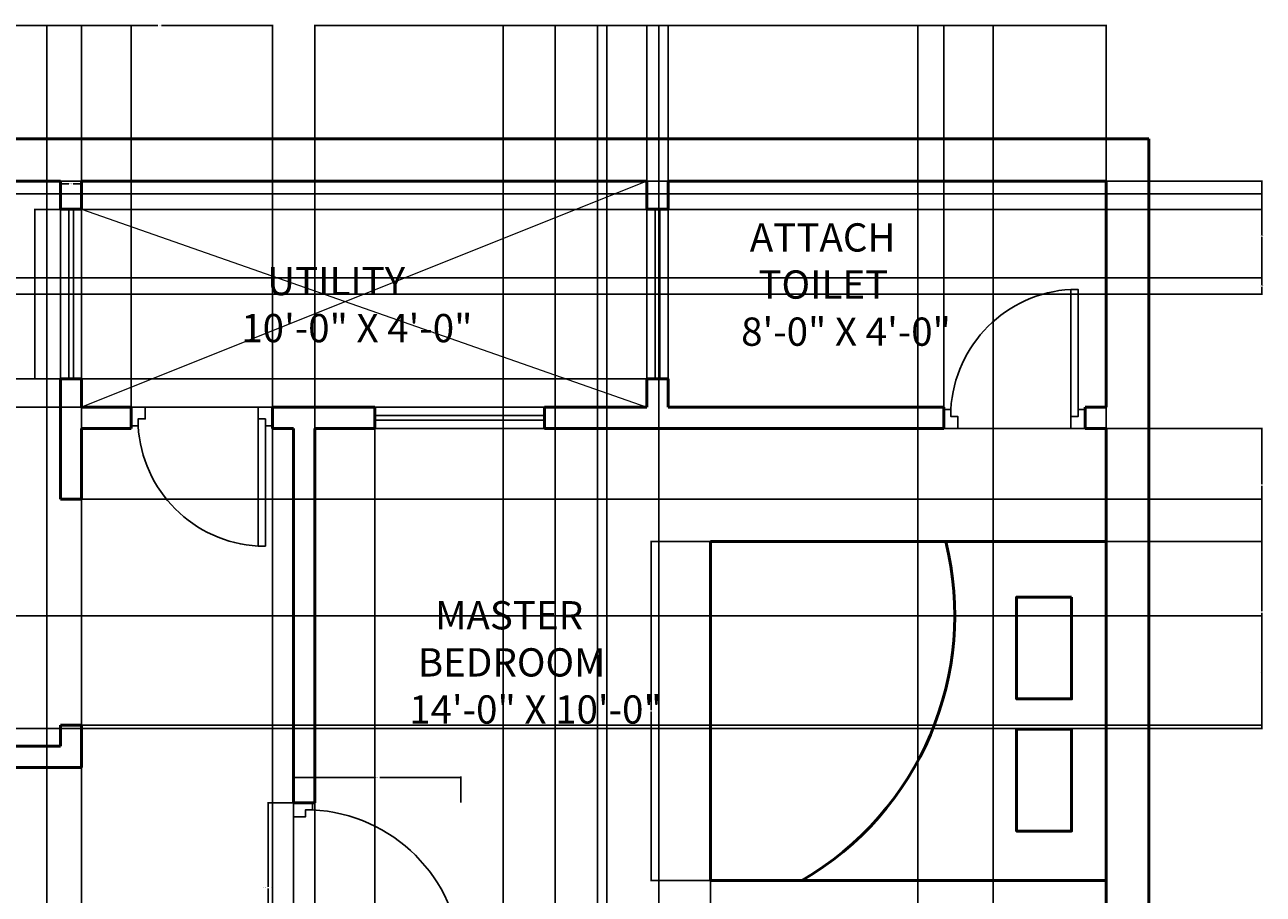
# Model space of a CAD drawing. Units: inches. Extents: x 2330 to 2739, y 947 to 1475.
# Tile 6 of 6: x 2476 to 2739, y 1291 to 1475. Entities that reach past the tile are written whole.
import ezdxf

# ---------------------------------------------------------------- set-up
doc = ezdxf.new("R2010")
doc.units = ezdxf.units.IN
for name, color, linetype, lineweight in [('A-ANNO-DIMS', 2, 'Continuous', 18), ('A-AREA-IDEN', 7, 'Continuous', 25), ('door', 150, 'Continuous', 25), ('furniture', 9, 'Continuous', 18), ('railing', 224, 'Continuous', 13), ('wall', 7, 'Continuous', 50), ('window', 40, 'Continuous', 25)]:
    doc.layers.add(name, color=color, linetype=linetype, lineweight=lineweight)
doc.styles.get("Standard").update_dxf_attribs({"font": 'arial.ttf'})
doc.dimstyles.get("Standard").update_dxf_attribs({"dimtxt": 0.18, "dimasz": 0.18, "dimexe": 0.18, "dimexo": 0.0625, "dimgap": 0.09, "dimtad": 0, "dimtih": 1, "dimtoh": 1, "dimdec": 4, "dimzin": 0, "dimdsep": 46, "dimtxsty": 'Standard', "dimcen": 0.09, "dimadec": 0, "dimazin": 0, "dimtfac": 1, "dimtdec": 4, "dimtofl": 0, "dimtmove": 0, "dimatfit": 3, "dimfxl": 1, "dimtolj": 1, "dimtzin": 0, "dimarcsym": 0})

# ---------------------------------------------------------------- blocks, each defined once
blk = doc.blocks.new('w3')
at = {"layer": 'window'}
for p, q in [((2833.35, 1386.77), (2833.35, 1350.77)), ((2834.35, 1386.77), (2834.35, 1350.77))]:
    blk.add_line(p, q, dxfattribs=at)
blk.add_lwpolyline([(2831.6, 1350.77), (2836.1, 1350.77), (2836.1, 1386.77), (2831.6, 1386.77)], close=True, dxfattribs=at)
blk = doc.blocks.new('d1')
at = {"layer": 'door'}
blk.add_line((2897.27, 1313.4), (2933.27, 1313.4), dxfattribs=at)
blk.add_lwpolyline([(2898.77, 1315.9), (2900.27, 1315.9), (2900.27, 1348.9), (2898.77, 1348.9)], close=True, dxfattribs=at)
for points in [[(2900.27, 1313.4), (2897.27, 1313.4), (2897.27, 1317.4), (2898.77, 1317.4), (2898.77, 1315.9), (2900.27, 1315.9), (2900.27, 1313.4)], [(2930.27, 1313.4), (2933.27, 1313.4), (2933.27, 1317.4), (2931.77, 1317.4), (2931.77, 1315.9), (2930.27, 1315.9), (2930.27, 1313.4)]]:
    blk.add_lwpolyline(points, dxfattribs=at)
blk.add_arc((2898.77, 1315.9), 33.03, 2.6026, 87.3974, dxfattribs=at)
blk = doc.blocks.new('d2')
at = {"layer": 'door'}
blk.add_line((2897.27, 1250.29), (2927.27, 1250.29), dxfattribs=at)
blk.add_lwpolyline([(2898.77, 1252.79), (2900.27, 1252.79), (2900.27, 1279.79), (2898.77, 1279.79)], close=True, dxfattribs=at)
for points in [[(2900.27, 1250.29), (2897.27, 1250.29), (2897.27, 1254.29), (2898.77, 1254.29), (2898.77, 1252.79), (2900.27, 1252.79), (2900.27, 1250.29)], [(2924.27, 1250.29), (2927.27, 1250.29), (2927.27, 1254.29), (2925.77, 1254.29), (2925.77, 1252.79), (2924.27, 1252.79), (2924.27, 1250.29)]]:
    blk.add_lwpolyline(points, dxfattribs=at)
blk.add_arc((2898.77, 1252.79), 27.04, 3.1798, 86.8202, dxfattribs=at)
blk = doc.blocks.new('BED')
at = {"layer": 'wall'}
for points in [[(2902.88, 1364.87), (2974.88, 1364.87), (2974.88, 1448.87), (2902.88, 1448.87)], [(2914.71, 1441.49), (2936.34, 1441.49), (2936.34, 1429.82), (2914.71, 1429.82)], [(2942.76, 1441.49), (2964.39, 1441.49), (2964.39, 1429.82), (2942.76, 1429.82)]]:
    blk.add_lwpolyline(points, close=True, dxfattribs=at)
blk.add_arc((2918.5, 1351.51), 65.2, 30.1485, 103.8594, dxfattribs=at)
blk = doc.blocks.new('*D10')
at = {"layer": 'A-ANNO-DIMS', "color": 0, "lineweight": -2, "transparency": 16777216}
for p, q in [((2483.62, 1436.28), (2478.1, 1436.28)), ((2478.28, 1436.1), (2478.28, 1418.47)), ((2478.28, 1400.46), (2478.28, 1418.1)), ((2483.62, 1400.28), (2478.1, 1400.28))]:
    blk.add_line(p, q, dxfattribs=at)
at = {"layer": 'A-ANNO-DIMS', "color": 0, "transparency": 16777216}
for points in [[(2478.25, 1436.1), (2478.31, 1436.1), (2478.28, 1436.28)], [(2478.25, 1400.46), (2478.31, 1400.46), (2478.28, 1400.28)]]:
    blk.add_solid(points, dxfattribs=at)
at = {"layer": 'Defpoints', "color": 0, "transparency": 16777216}
for p in [(2478.28, 1436.28), (2483.68, 1436.28), (2483.68, 1400.28)]:
    blk.add_point(p, dxfattribs=at)
at = {"layer": 'A-ANNO-DIMS', "color": 0, "transparency": 16777216, "insert": (2478.28, 1418.28), "char_height": 0.18, "attachment_point": 5}
blk.add_mtext('\\A1;WINDOW W3 36 TYP.', dxfattribs=at)
blk = doc.blocks.new('*D11')
at = {"layer": 'A-ANNO-DIMS', "color": 0, "lineweight": -2, "transparency": 16777216}
for p, q in [((2483.68, 1436.34), (2483.68, 1441.86)), ((2483.86, 1441.68), (2485.47, 1441.68)), ((2488, 1441.68), (2486.39, 1441.68)), ((2488.18, 1436.34), (2488.18, 1441.86))]:
    blk.add_line(p, q, dxfattribs=at)
at = {"layer": 'A-ANNO-DIMS', "color": 0, "transparency": 16777216}
for points in [[(2483.86, 1441.71), (2483.86, 1441.65), (2483.68, 1441.68)], [(2488, 1441.71), (2488, 1441.65), (2488.18, 1441.68)]]:
    blk.add_solid(points, dxfattribs=at)
at = {"layer": 'Defpoints', "color": 0, "transparency": 16777216}
for p in [(2488.18, 1441.68), (2483.68, 1436.28), (2488.18, 1436.28)]:
    blk.add_point(p, dxfattribs=at)
at = {"layer": 'A-ANNO-DIMS', "color": 0, "transparency": 16777216, "insert": (2485.93, 1441.68), "char_height": 0.18, "attachment_point": 5}
blk.add_mtext('\\A1;5 TYP.', dxfattribs=at)
blk = doc.blocks.new('*D16')
at = {"layer": 'A-ANNO-DIMS', "color": 0, "lineweight": -2, "transparency": 16777216}
for p, q in [((2533.12, 1310.28), (2527.6, 1310.28)), ((2527.78, 1310.1), (2527.78, 1292.47)), ((2527.78, 1274.46), (2527.78, 1292.1)), ((2533.12, 1274.28), (2527.6, 1274.28))]:
    blk.add_line(p, q, dxfattribs=at)
at = {"layer": 'A-ANNO-DIMS', "color": 0, "transparency": 16777216}
for points in [[(2527.75, 1310.1), (2527.81, 1310.1), (2527.78, 1310.28)], [(2527.75, 1274.46), (2527.81, 1274.46), (2527.78, 1274.28)]]:
    blk.add_solid(points, dxfattribs=at)
at = {"layer": 'Defpoints', "color": 0, "transparency": 16777216}
for p in [(2527.78, 1310.28), (2533.18, 1310.28), (2533.18, 1274.28)]:
    blk.add_point(p, dxfattribs=at)
at = {"layer": 'A-ANNO-DIMS', "color": 0, "transparency": 16777216, "insert": (2527.78, 1292.28), "char_height": 0.18, "attachment_point": 5}
blk.add_mtext('\\A1;DOOR D1 36 TYP.', dxfattribs=at)
blk = doc.blocks.new('*D17')
at = {"layer": 'A-ANNO-DIMS', "color": 0, "lineweight": -2, "transparency": 16777216}
for p, q in [((2533.18, 1310.34), (2533.18, 1315.86)), ((2533.36, 1315.68), (2550.4, 1315.68)), ((2568.5, 1315.68), (2551.46, 1315.68)), ((2568.68, 1310.34), (2568.68, 1315.86))]:
    blk.add_line(p, q, dxfattribs=at)
at = {"layer": 'A-ANNO-DIMS', "color": 0, "transparency": 16777216}
for points in [[(2533.36, 1315.71), (2533.36, 1315.65), (2533.18, 1315.68)], [(2568.5, 1315.71), (2568.5, 1315.65), (2568.68, 1315.68)]]:
    blk.add_solid(points, dxfattribs=at)
at = {"layer": 'Defpoints', "color": 0, "transparency": 16777216}
for p in [(2568.68, 1315.68), (2533.18, 1310.28), (2568.68, 1310.28)]:
    blk.add_point(p, dxfattribs=at)
at = {"layer": 'A-ANNO-DIMS', "color": 0, "transparency": 16777216, "insert": (2550.93, 1315.68), "char_height": 0.18, "attachment_point": 5}
blk.add_mtext('\\A1;36 TYP.', dxfattribs=at)
blk = doc.blocks.new('*D18')
at = {"layer": 'A-ANNO-DIMS', "color": 0, "lineweight": -2, "transparency": 16777216}
for p, q in [((2621.68, 1293.72), (2621.68, 1281)), ((2705.68, 1293.72), (2705.68, 1281)), ((2621.86, 1281.18), (2662.86, 1281.18)), ((2705.5, 1281.18), (2664.5, 1281.18))]:
    blk.add_line(p, q, dxfattribs=at)
at = {"layer": 'A-ANNO-DIMS', "color": 0, "transparency": 16777216}
for points in [[(2621.86, 1281.21), (2621.86, 1281.15), (2621.68, 1281.18)], [(2705.5, 1281.21), (2705.5, 1281.15), (2705.68, 1281.18)]]:
    blk.add_solid(points, dxfattribs=at)
at = {"layer": 'Defpoints', "color": 0, "transparency": 16777216}
for p in [(2621.68, 1293.78), (2705.68, 1293.78), (2705.68, 1281.18)]:
    blk.add_point(p, dxfattribs=at)
at = {"layer": 'A-ANNO-DIMS', "color": 0, "transparency": 16777216, "insert": (2663.68, 1281.18), "char_height": 0.18, "attachment_point": 5}
blk.add_mtext('\\A1;BED 84 TYP.', dxfattribs=at)
blk = doc.blocks.new('*D19')
at = {"layer": 'A-ANNO-DIMS', "color": 0, "lineweight": -2, "transparency": 16777216}
for p, q in [((2621.62, 1365.78), (2608.9, 1365.78)), ((2609.08, 1365.6), (2609.08, 1329.96)), ((2609.08, 1293.96), (2609.08, 1329.6)), ((2621.62, 1293.78), (2608.9, 1293.78))]:
    blk.add_line(p, q, dxfattribs=at)
at = {"layer": 'A-ANNO-DIMS', "color": 0, "transparency": 16777216}
for points in [[(2609.05, 1365.6), (2609.11, 1365.6), (2609.08, 1365.78)], [(2609.05, 1293.96), (2609.11, 1293.96), (2609.08, 1293.78)]]:
    blk.add_solid(points, dxfattribs=at)
at = {"layer": 'Defpoints', "color": 0, "transparency": 16777216}
for p in [(2621.68, 1365.78), (2609.08, 1293.78), (2621.68, 1293.78)]:
    blk.add_point(p, dxfattribs=at)
at = {"layer": 'A-ANNO-DIMS', "color": 0, "transparency": 16777216, "insert": (2609.08, 1329.78), "char_height": 0.18, "attachment_point": 5}
blk.add_mtext('\\A1;72 TYP.', dxfattribs=at)
blk = doc.blocks.new('*D27')
at = {"layer": 'A-ANNO-DIMS', "color": 0, "lineweight": -2, "transparency": 16777216}
for p, q in [((2537.68, 980.34), (2537.68, 1475.46)), ((2537.86, 1475.28), (2567.46, 1475.28)), ((2597.5, 1475.28), (2567.9, 1475.28)), ((2597.68, 980.34), (2597.68, 1475.46))]:
    blk.add_line(p, q, dxfattribs=at)
at = {"layer": 'A-ANNO-DIMS', "color": 0, "transparency": 16777216}
for points in [[(2537.86, 1475.31), (2537.86, 1475.25), (2537.68, 1475.28)], [(2597.5, 1475.31), (2597.5, 1475.25), (2597.68, 1475.28)]]:
    blk.add_solid(points, dxfattribs=at)
at = {"layer": 'Defpoints', "color": 0, "transparency": 16777216}
for p in [(2597.68, 1475.28), (2537.68, 980.28), (2597.68, 980.28)]:
    blk.add_point(p, dxfattribs=at)
at = {"layer": 'A-ANNO-DIMS', "color": 0, "transparency": 16777216, "insert": (2567.68, 1475.28), "char_height": 0.18, "attachment_point": 5}
blk.add_mtext('\\A1;60', dxfattribs=at)
blk = doc.blocks.new('*D29')
at = {"layer": 'A-ANNO-DIMS', "color": 0, "lineweight": -2, "transparency": 16777216}
for p, q in [((2705.74, 1389.78), (2738.86, 1389.78)), ((2738.68, 1389.6), (2738.68, 1377.96)), ((2738.68, 1365.96), (2738.68, 1377.6)), ((2705.74, 1365.78), (2738.86, 1365.78))]:
    blk.add_line(p, q, dxfattribs=at)
at = {"layer": 'A-ANNO-DIMS', "color": 0, "transparency": 16777216}
for points in [[(2738.65, 1389.6), (2738.71, 1389.6), (2738.68, 1389.78)], [(2738.65, 1365.96), (2738.71, 1365.96), (2738.68, 1365.78)]]:
    blk.add_solid(points, dxfattribs=at)
at = {"layer": 'Defpoints', "color": 0, "transparency": 16777216}
for p in [(2705.68, 1389.78), (2705.68, 1365.78), (2738.68, 1365.78)]:
    blk.add_point(p, dxfattribs=at)
at = {"layer": 'A-ANNO-DIMS', "color": 0, "transparency": 16777216, "insert": (2738.68, 1377.78), "char_height": 0.18, "attachment_point": 5}
blk.add_mtext('\\A1;24', dxfattribs=at)
blk = doc.blocks.new('*D34')
at = {"layer": 'A-ANNO-DIMS', "color": 0, "lineweight": -2, "transparency": 16777216}
for p, q in [((2449.93, 1139.34), (2449.93, 1475.46)), ((2450.11, 1475.28), (2468.66, 1475.28)), ((2488, 1475.28), (2469.45, 1475.28)), ((2488.18, 1139.34), (2488.18, 1475.46))]:
    blk.add_line(p, q, dxfattribs=at)
at = {"layer": 'A-ANNO-DIMS', "color": 0, "transparency": 16777216}
for points in [[(2450.11, 1475.31), (2450.11, 1475.25), (2449.93, 1475.28)], [(2488, 1475.31), (2488, 1475.25), (2488.18, 1475.28)]]:
    blk.add_solid(points, dxfattribs=at)
at = {"layer": 'Defpoints', "color": 0, "transparency": 16777216}
for p in [(2488.18, 1475.28), (2449.93, 1139.28), (2488.18, 1139.28)]:
    blk.add_point(p, dxfattribs=at)
at = {"layer": 'A-ANNO-DIMS', "color": 0, "transparency": 16777216, "insert": (2469.05, 1475.28), "char_height": 0.18, "attachment_point": 5}
blk.add_mtext('\\A1;38.25', dxfattribs=at)
blk = doc.blocks.new('*D35')
at = {"layer": 'A-ANNO-DIMS', "color": 0, "lineweight": -2, "transparency": 16777216}
for p, q in [((2488.18, 1394.34), (2488.18, 1475.46)), ((2488.36, 1475.28), (2493.11, 1475.28)), ((2498.5, 1475.28), (2493.74, 1475.28)), ((2498.68, 1394.34), (2498.68, 1475.46))]:
    blk.add_line(p, q, dxfattribs=at)
at = {"layer": 'A-ANNO-DIMS', "color": 0, "transparency": 16777216}
for points in [[(2488.36, 1475.31), (2488.36, 1475.25), (2488.18, 1475.28)], [(2498.5, 1475.31), (2498.5, 1475.25), (2498.68, 1475.28)]]:
    blk.add_solid(points, dxfattribs=at)
at = {"layer": 'Defpoints', "color": 0, "transparency": 16777216}
for p in [(2498.68, 1475.28), (2488.18, 1394.28), (2498.68, 1394.28)]:
    blk.add_point(p, dxfattribs=at)
at = {"layer": 'A-ANNO-DIMS', "color": 0, "transparency": 16777216, "insert": (2493.43, 1475.28), "char_height": 0.18, "attachment_point": 5}
blk.add_mtext('\\A1;10.5', dxfattribs=at)
blk = doc.blocks.new('*D36')
at = {"layer": 'A-ANNO-DIMS', "color": 0, "lineweight": -2, "transparency": 16777216}
for p, q in [((2528.68, 1394.22), (2528.68, 947.1)), ((2550.43, 1394.22), (2550.43, 947.1)), ((2528.86, 947.28), (2539.16, 947.28)), ((2550.25, 947.28), (2539.95, 947.28))]:
    blk.add_line(p, q, dxfattribs=at)
at = {"layer": 'A-ANNO-DIMS', "color": 0, "transparency": 16777216}
for points in [[(2528.86, 947.31), (2528.86, 947.25), (2528.68, 947.28)], [(2550.25, 947.31), (2550.25, 947.25), (2550.43, 947.28)]]:
    blk.add_solid(points, dxfattribs=at)
at = {"layer": 'Defpoints', "color": 0, "transparency": 16777216}
for p in [(2528.68, 1394.28), (2550.43, 1394.28), (2550.43, 947.28)]:
    blk.add_point(p, dxfattribs=at)
at = {"layer": 'A-ANNO-DIMS', "color": 0, "transparency": 16777216, "insert": (2539.55, 947.28), "char_height": 0.18, "attachment_point": 5}
blk.add_mtext('\\A1;21.75', dxfattribs=at)
blk = doc.blocks.new('*D37')
at = {"layer": 'A-ANNO-DIMS', "color": 0, "lineweight": -2, "transparency": 16777216}
for p, q in [((2608.18, 1442.34), (2608.18, 1475.46)), ((2608.36, 1475.28), (2610.17, 1475.28)), ((2612.5, 1475.28), (2610.69, 1475.28)), ((2612.68, 1442.34), (2612.68, 1475.46))]:
    blk.add_line(p, q, dxfattribs=at)
at = {"layer": 'A-ANNO-DIMS', "color": 0, "transparency": 16777216}
for points in [[(2608.36, 1475.31), (2608.36, 1475.25), (2608.18, 1475.28)], [(2612.5, 1475.31), (2612.5, 1475.25), (2612.68, 1475.28)]]:
    blk.add_solid(points, dxfattribs=at)
at = {"layer": 'Defpoints', "color": 0, "transparency": 16777216}
for p in [(2608.18, 1475.28), (2608.18, 1442.28), (2612.68, 1442.28)]:
    blk.add_point(p, dxfattribs=at)
at = {"layer": 'A-ANNO-DIMS', "color": 0, "transparency": 16777216, "insert": (2610.43, 1475.28), "char_height": 0.18, "attachment_point": 5}
blk.add_mtext('\\A1;4.5', dxfattribs=at)
blk = doc.blocks.new('*D38')
at = {"layer": 'A-ANNO-DIMS', "color": 0, "lineweight": -2, "transparency": 16777216}
for p, q in [((2537.68, 1134.84), (2537.68, 1475.46)), ((2537.86, 1475.28), (2562.98, 1475.28)), ((2588.5, 1475.28), (2563.38, 1475.28)), ((2588.68, 1134.84), (2588.68, 1475.46))]:
    blk.add_line(p, q, dxfattribs=at)
at = {"layer": 'A-ANNO-DIMS', "color": 0, "transparency": 16777216}
for points in [[(2537.86, 1475.31), (2537.86, 1475.25), (2537.68, 1475.28)], [(2588.5, 1475.31), (2588.5, 1475.25), (2588.68, 1475.28)]]:
    blk.add_solid(points, dxfattribs=at)
at = {"layer": 'Defpoints', "color": 0, "transparency": 16777216}
for p in [(2588.68, 1475.28), (2537.68, 1134.78), (2588.68, 1134.78)]:
    blk.add_point(p, dxfattribs=at)
at = {"layer": 'A-ANNO-DIMS', "color": 0, "transparency": 16777216, "insert": (2563.18, 1475.28), "char_height": 0.18, "attachment_point": 5}
blk.add_mtext('\\A1;51', dxfattribs=at)
blk = doc.blocks.new('*D41')
at = {"layer": 'A-ANNO-DIMS', "color": 0, "lineweight": -2, "transparency": 16777216}
for p, q in [((2612.68, 1394.34), (2612.68, 1475.46)), ((2612.86, 1475.28), (2641.6, 1475.28)), ((2671, 1475.28), (2642.25, 1475.28)), ((2671.18, 1394.34), (2671.18, 1475.46))]:
    blk.add_line(p, q, dxfattribs=at)
at = {"layer": 'A-ANNO-DIMS', "color": 0, "transparency": 16777216}
for points in [[(2612.86, 1475.31), (2612.86, 1475.25), (2612.68, 1475.28)], [(2671, 1475.31), (2671, 1475.25), (2671.18, 1475.28)]]:
    blk.add_solid(points, dxfattribs=at)
at = {"layer": 'Defpoints', "color": 0, "transparency": 16777216}
for p in [(2612.68, 1475.28), (2612.68, 1394.28), (2671.18, 1394.28)]:
    blk.add_point(p, dxfattribs=at)
at = {"layer": 'A-ANNO-DIMS', "color": 0, "transparency": 16777216, "insert": (2641.93, 1475.28), "char_height": 0.18, "attachment_point": 5}
blk.add_mtext('\\A1;58.5', dxfattribs=at)
blk = doc.blocks.new('*D62')
at = {"layer": 'A-ANNO-DIMS', "color": 0, "lineweight": -2, "transparency": 16777216}
for p, q in [((2426.7, 1439.54), (2738.86, 1439.54)), ((2738.68, 1439.36), (2738.68, 1430.83)), ((2738.68, 1421.95), (2738.68, 1430.47)), ((2426.7, 1421.77), (2738.86, 1421.77))]:
    blk.add_line(p, q, dxfattribs=at)
at = {"layer": 'A-ANNO-DIMS', "color": 0, "transparency": 16777216}
for points in [[(2738.65, 1439.36), (2738.71, 1439.36), (2738.68, 1439.54)], [(2738.65, 1421.95), (2738.71, 1421.95), (2738.68, 1421.77)]]:
    blk.add_solid(points, dxfattribs=at)
at = {"layer": 'Defpoints', "color": 0, "transparency": 16777216}
for p in [(2426.64, 1439.54), (2738.68, 1439.54), (2426.64, 1421.77)]:
    blk.add_point(p, dxfattribs=at)
at = {"layer": 'A-ANNO-DIMS', "color": 0, "transparency": 16777216, "insert": (2738.68, 1430.65), "char_height": 0.18, "attachment_point": 5}
blk.add_mtext('\\A1;17.77', dxfattribs=at)
blk = doc.blocks.new('*D64')
at = {"layer": 'A-ANNO-DIMS', "color": 0, "lineweight": -2, "transparency": 16777216}
for p, q in [((2426.7, 1421.77), (2738.86, 1421.77)), ((2738.68, 1421.59), (2738.68, 1420.21)), ((2738.68, 1418.46), (2738.68, 1419.84)), ((2443.26, 1418.28), (2738.86, 1418.28))]:
    blk.add_line(p, q, dxfattribs=at)
at = {"layer": 'A-ANNO-DIMS', "color": 0, "transparency": 16777216}
for points in [[(2738.65, 1421.59), (2738.71, 1421.59), (2738.68, 1421.77)], [(2738.65, 1418.46), (2738.71, 1418.46), (2738.68, 1418.28)]]:
    blk.add_solid(points, dxfattribs=at)
at = {"layer": 'Defpoints', "color": 0, "transparency": 16777216}
for p in [(2426.64, 1421.77), (2443.2, 1418.28), (2738.68, 1418.28)]:
    blk.add_point(p, dxfattribs=at)
at = {"layer": 'A-ANNO-DIMS', "color": 0, "transparency": 16777216, "insert": (2738.68, 1420.03), "char_height": 0.18, "attachment_point": 5}
blk.add_mtext('\\A1;3.487', dxfattribs=at)
blk = doc.blocks.new('*D68')
at = {"layer": 'A-ANNO-DIMS', "color": 0, "lineweight": -2, "transparency": 16777216}
for p, q in [((2483.74, 1374.78), (2738.86, 1374.78)), ((2738.68, 1374.6), (2738.68, 1350.96)), ((2738.68, 1326.96), (2738.68, 1350.6)), ((2483.74, 1326.78), (2738.86, 1326.78))]:
    blk.add_line(p, q, dxfattribs=at)
at = {"layer": 'A-ANNO-DIMS', "color": 0, "transparency": 16777216}
for points in [[(2738.65, 1374.6), (2738.71, 1374.6), (2738.68, 1374.78)], [(2738.65, 1326.96), (2738.71, 1326.96), (2738.68, 1326.78)]]:
    blk.add_solid(points, dxfattribs=at)
at = {"layer": 'Defpoints', "color": 0, "transparency": 16777216}
for p in [(2483.68, 1374.78), (2738.68, 1374.78), (2483.68, 1326.78)]:
    blk.add_point(p, dxfattribs=at)
at = {"layer": 'A-ANNO-DIMS', "color": 0, "transparency": 16777216, "insert": (2738.68, 1350.78), "char_height": 0.18, "attachment_point": 5}
blk.add_mtext('\\A1;48', dxfattribs=at)
blk = doc.blocks.new('*D69')
at = {"layer": 'A-ANNO-DIMS', "color": 0, "lineweight": -2, "transparency": 16777216}
for p, q in [((2483.74, 1442.28), (2738.86, 1442.28)), ((2738.68, 1442.1), (2738.68, 1439.46)), ((2738.68, 1436.46), (2738.68, 1439.1)), ((2483.74, 1436.28), (2738.86, 1436.28))]:
    blk.add_line(p, q, dxfattribs=at)
at = {"layer": 'A-ANNO-DIMS', "color": 0, "transparency": 16777216}
for points in [[(2738.65, 1442.1), (2738.71, 1442.1), (2738.68, 1442.28)], [(2738.65, 1436.46), (2738.71, 1436.46), (2738.68, 1436.28)]]:
    blk.add_solid(points, dxfattribs=at)
at = {"layer": 'Defpoints', "color": 0, "transparency": 16777216}
for p in [(2483.68, 1442.28), (2483.68, 1436.28), (2738.68, 1436.28)]:
    blk.add_point(p, dxfattribs=at)
at = {"layer": 'A-ANNO-DIMS', "color": 0, "transparency": 16777216, "insert": (2738.68, 1439.28), "char_height": 0.18, "attachment_point": 5}
blk.add_mtext('\\A1;6', dxfattribs=at)
blk = doc.blocks.new('*D71')
at = {"layer": 'A-ANNO-DIMS', "color": 0, "lineweight": -2, "transparency": 16777216}
for p, q in [((2392.26, 1349.96), (2738.86, 1349.96)), ((2738.68, 1349.78), (2738.68, 1338.17)), ((2738.68, 1326.21), (2738.68, 1337.81)), ((2392.26, 1326.03), (2738.86, 1326.03))]:
    blk.add_line(p, q, dxfattribs=at)
at = {"layer": 'A-ANNO-DIMS', "color": 0, "transparency": 16777216}
for points in [[(2738.65, 1349.78), (2738.71, 1349.78), (2738.68, 1349.96)], [(2738.65, 1326.21), (2738.71, 1326.21), (2738.68, 1326.03)]]:
    blk.add_solid(points, dxfattribs=at)
at = {"layer": 'Defpoints', "color": 0, "transparency": 16777216}
for p in [(2392.19, 1349.96), (2738.68, 1349.96), (2392.19, 1326.03)]:
    blk.add_point(p, dxfattribs=at)
at = {"layer": 'A-ANNO-DIMS', "color": 0, "transparency": 16777216, "insert": (2738.68, 1337.99), "char_height": 0.18, "attachment_point": 5}
blk.add_mtext('\\A1;23.93', dxfattribs=at)
blk = doc.blocks.new('*D72')
at = {"layer": 'A-ANNO-DIMS', "color": 0, "lineweight": -2, "transparency": 16777216}
for p, q in [((2599.68, 1187.34), (2599.68, 1475.46)), ((2599.86, 1475.28), (2604.99, 1475.28)), ((2610.5, 1475.28), (2605.37, 1475.28)), ((2610.68, 1187.34), (2610.68, 1475.46))]:
    blk.add_line(p, q, dxfattribs=at)
at = {"layer": 'A-ANNO-DIMS', "color": 0, "transparency": 16777216}
for points in [[(2599.86, 1475.31), (2599.86, 1475.25), (2599.68, 1475.28)], [(2610.5, 1475.31), (2610.5, 1475.25), (2610.68, 1475.28)]]:
    blk.add_solid(points, dxfattribs=at)
at = {"layer": 'Defpoints', "color": 0, "transparency": 16777216}
for p in [(2610.68, 1475.28), (2599.68, 1187.28), (2610.68, 1187.28)]:
    blk.add_point(p, dxfattribs=at)
at = {"layer": 'A-ANNO-DIMS', "color": 0, "transparency": 16777216, "insert": (2605.18, 1475.28), "char_height": 0.18, "attachment_point": 5}
blk.add_mtext('\\A1;11', dxfattribs=at)
blk = doc.blocks.new('*D75')
at = {"layer": 'A-ANNO-DIMS', "color": 0, "lineweight": -2, "transparency": 16777216}
for p, q in [((2665.68, 1187.34), (2665.68, 1475.46)), ((2665.86, 1475.28), (2685.46, 1475.28)), ((2705.5, 1475.28), (2685.9, 1475.28)), ((2705.68, 1187.34), (2705.68, 1475.46))]:
    blk.add_line(p, q, dxfattribs=at)
at = {"layer": 'A-ANNO-DIMS', "color": 0, "transparency": 16777216}
for points in [[(2665.86, 1475.31), (2665.86, 1475.25), (2665.68, 1475.28)], [(2705.5, 1475.31), (2705.5, 1475.25), (2705.68, 1475.28)]]:
    blk.add_solid(points, dxfattribs=at)
at = {"layer": 'Defpoints', "color": 0, "transparency": 16777216}
for p in [(2705.68, 1475.28), (2665.68, 1187.28), (2705.68, 1187.28)]:
    blk.add_point(p, dxfattribs=at)
at = {"layer": 'A-ANNO-DIMS', "color": 0, "transparency": 16777216, "insert": (2685.68, 1475.28), "char_height": 0.18, "attachment_point": 5}
blk.add_mtext('\\A1;40', dxfattribs=at)
blk = doc.blocks.new('*D76')
at = {"layer": 'A-ANNO-DIMS', "color": 0, "lineweight": -2, "transparency": 16777216}
for p, q in [((2577.68, 1265.34), (2577.68, 1475.46)), ((2577.86, 1475.28), (2621.46, 1475.28)), ((2665.5, 1475.28), (2621.9, 1475.28)), ((2665.68, 1265.34), (2665.68, 1475.46))]:
    blk.add_line(p, q, dxfattribs=at)
at = {"layer": 'A-ANNO-DIMS', "color": 0, "transparency": 16777216}
for points in [[(2577.86, 1475.31), (2577.86, 1475.25), (2577.68, 1475.28)], [(2665.5, 1475.31), (2665.5, 1475.25), (2665.68, 1475.28)]]:
    blk.add_solid(points, dxfattribs=at)
at = {"layer": 'Defpoints', "color": 0, "transparency": 16777216}
for p in [(2665.68, 1475.28), (2577.68, 1265.28), (2665.68, 1265.28)]:
    blk.add_point(p, dxfattribs=at)
at = {"layer": 'A-ANNO-DIMS', "color": 0, "transparency": 16777216, "insert": (2621.68, 1475.28), "char_height": 0.18, "attachment_point": 5}
blk.add_mtext('\\A1;88', dxfattribs=at)
blk = doc.blocks.new('*D78')
at = {"layer": 'A-ANNO-DIMS', "color": 0, "lineweight": -2, "transparency": 16777216}
for p, q in [((2681.68, 1182.84), (2681.68, 1475.46)), ((2681.86, 1475.28), (2693.46, 1475.28)), ((2705.5, 1475.28), (2693.9, 1475.28)), ((2705.68, 1182.84), (2705.68, 1475.46))]:
    blk.add_line(p, q, dxfattribs=at)
at = {"layer": 'A-ANNO-DIMS', "color": 0, "transparency": 16777216}
for points in [[(2681.86, 1475.31), (2681.86, 1475.25), (2681.68, 1475.28)], [(2705.5, 1475.31), (2705.5, 1475.25), (2705.68, 1475.28)]]:
    blk.add_solid(points, dxfattribs=at)
at = {"layer": 'Defpoints', "color": 0, "transparency": 16777216}
for p in [(2705.68, 1475.28), (2681.68, 1182.78), (2705.68, 1182.78)]:
    blk.add_point(p, dxfattribs=at)
at = {"layer": 'A-ANNO-DIMS', "color": 0, "transparency": 16777216, "insert": (2693.68, 1475.28), "char_height": 0.18, "attachment_point": 5}
blk.add_mtext('\\A1;24', dxfattribs=at)
blk = doc.blocks.new('*D79')
at = {"layer": 'A-ANNO-DIMS', "color": 0, "lineweight": -2, "transparency": 16777216}
for p, q in [((2608.12, 1400.28), (2330.5, 1400.28)), ((2330.68, 1400.1), (2330.68, 1397.46)), ((2330.68, 1394.46), (2330.68, 1397.1)), ((2608.12, 1394.28), (2330.5, 1394.28))]:
    blk.add_line(p, q, dxfattribs=at)
at = {"layer": 'A-ANNO-DIMS', "color": 0, "transparency": 16777216}
for points in [[(2330.65, 1400.1), (2330.71, 1400.1), (2330.68, 1400.28)], [(2330.65, 1394.46), (2330.71, 1394.46), (2330.68, 1394.28)]]:
    blk.add_solid(points, dxfattribs=at)
at = {"layer": 'Defpoints', "color": 0, "transparency": 16777216}
for p in [(2608.18, 1400.28), (2330.68, 1394.28), (2608.18, 1394.28)]:
    blk.add_point(p, dxfattribs=at)
at = {"layer": 'A-ANNO-DIMS', "color": 0, "transparency": 16777216, "insert": (2330.68, 1397.28), "char_height": 0.18, "attachment_point": 5}
blk.add_mtext('\\A1;6', dxfattribs=at)
blk = doc.blocks.new('*D80')
at = {"layer": 'A-ANNO-DIMS', "color": 0, "lineweight": -2, "transparency": 16777216}
for p, q in [((2480.81, 1118.34), (2480.81, 1475.46)), ((2480.99, 1475.28), (2504.34, 1475.28)), ((2528.5, 1475.28), (2505.14, 1475.28)), ((2528.68, 1118.34), (2528.68, 1475.46))]:
    blk.add_line(p, q, dxfattribs=at)
at = {"layer": 'A-ANNO-DIMS', "color": 0, "transparency": 16777216}
for points in [[(2480.99, 1475.31), (2480.99, 1475.25), (2480.81, 1475.28)], [(2528.5, 1475.31), (2528.5, 1475.25), (2528.68, 1475.28)]]:
    blk.add_solid(points, dxfattribs=at)
at = {"layer": 'Defpoints', "color": 0, "transparency": 16777216}
for p in [(2528.68, 1475.28), (2480.81, 1118.28), (2528.68, 1118.28)]:
    blk.add_point(p, dxfattribs=at)
at = {"layer": 'A-ANNO-DIMS', "color": 0, "transparency": 16777216, "insert": (2504.74, 1475.28), "char_height": 0.18, "attachment_point": 5}
blk.add_mtext('\\A1;47.87', dxfattribs=at)

msp = doc.modelspace()

# ---------------------------------------------------------------- linework, layer by layer
at = {"layer": 'railing'}
for p, q in [((2608.1781, 1442.2823), (2488.1781, 1394.2823)), ((2488.1781, 1436.2823), (2608.1781, 1394.2823))]:
    msp.add_line(p, q, dxfattribs=at)
at = {"layer": 'wall'}
for p, q in [((2714.6781, 1451.2823), (2354.6781, 1451.2823)), ((2714.6781, 971.2823), (2714.6781, 1451.2823)), ((2483.6781, 1442.2823), (2363.6781, 1442.2823)), ((2483.6781, 1442.2823), (2483.6781, 1436.2823)), ((2488.1781, 1442.2823), (2488.1781, 1436.2823)), ((2608.1781, 1442.2823), (2488.1781, 1442.2823)), ((2608.1781, 1442.2823), (2608.1781, 1436.2823)), ((2705.6781, 1442.2823), (2612.6781, 1442.2823)), ((2612.6781, 1442.2823), (2612.6781, 1436.2823)), ((2705.6781, 1394.2823), (2705.6781, 1442.2823)), ((2488.1781, 1436.2823), (2483.6781, 1436.2823)), ((2608.1781, 1436.2823), (2612.6781, 1436.2823)), ((2488.1781, 1400.2823), (2483.6781, 1400.2823)), ((2483.6781, 1400.2823), (2483.6781, 1374.7823)), ((2488.1781, 1400.2823), (2488.1781, 1394.2823)), ((2608.1781, 1400.2823), (2612.6781, 1400.2823)), ((2608.1781, 1400.2823), (2608.1781, 1394.2823)), ((2612.6781, 1400.2823), (2612.6781, 1394.2823)), ((2498.6781, 1394.2823), (2488.1781, 1394.2823)), ((2498.6781, 1389.7823), (2498.6781, 1394.2823)), ((2528.6781, 1389.7823), (2528.6781, 1394.2823)), ((2550.4281, 1394.2823), (2528.6781, 1394.2823)), ((2550.4281, 1394.2823), (2550.4281, 1389.7823)), ((2608.1781, 1394.2823), (2586.4281, 1394.2823)), ((2586.4281, 1394.2823), (2586.4281, 1389.7823)), ((2671.1781, 1394.2823), (2612.6781, 1394.2823)), ((2671.1781, 1389.7823), (2671.1781, 1394.2823)), ((2705.6781, 1394.2823), (2701.1781, 1394.2823)), ((2701.1781, 1389.7823), (2701.1781, 1394.2823)), ((2488.1781, 1389.7823), (2488.1781, 1374.7823)), ((2498.6781, 1389.7823), (2488.1781, 1389.7823)), ((2533.1781, 1389.7823), (2528.6781, 1389.7823)), ((2533.1781, 1310.2823), (2533.1781, 1389.7823)), ((2550.4281, 1389.7823), (2537.6781, 1389.7823)), ((2537.6781, 1310.2823), (2537.6781, 1389.7823)), ((2671.1781, 1389.7823), (2586.4281, 1389.7823)), ((2705.6781, 1389.7823), (2701.1781, 1389.7823)), ((2705.6781, 1269.7823), (2705.6781, 1389.7823)), ((2488.1781, 1374.7823), (2483.6781, 1374.7823)), ((2488.1781, 1326.7823), (2483.6781, 1326.7823)), ((2483.6781, 1326.7823), (2483.6781, 1322.2823)), ((2488.1781, 1326.7823), (2488.1781, 1317.7823)), ((2483.6781, 1322.2823), (2363.6781, 1322.2823)), ((2488.1781, 1317.7823), (2363.6781, 1317.7823)), ((2537.6781, 1310.2823), (2533.1781, 1310.2823))]:
    msp.add_line(p, q, dxfattribs=at)

# ---------------------------------------------------------------- block references
at = {"layer": 'door', "xscale": -1}
msp.add_blockref('d2', (5598.4472, 139.4913), dxfattribs=at)
at = {"layer": 'door', "rotation": 180}
msp.add_blockref('d2', (5425.9472, 2644.5733), dxfattribs=at)
at = {"layer": 'door', "xscale": -1, "rotation": 270}
msp.add_blockref('d1', (1219.7792, -1622.9868), dxfattribs=at)
at = {"layer": 'furniture', "rotation": 270}
msp.add_blockref('BED', (1256.8054, 4268.6666), dxfattribs=at)
at = {"layer": 'window'}
for p in [(-347.9186, 49.508), (-223.4186, 49.508)]:
    msp.add_blockref('w3', p, dxfattribs=at)
at = {"layer": 'window', "rotation": 270}
msp.add_blockref('w3', (1199.6539, 4225.879), dxfattribs=at)

# ---------------------------------------------------------------- texts
at = {"layer": 'A-AREA-IDEN', "char_height": 6, "attachment_point": 1}
for s, insert in [('   ATTACH\\P    TOILET\\P  8\'-0" X 4\'-0"', (2624.4983, 1433.3165)), ('   UTILITY\\P10\'-0" X 4\'-0"', (2522.0662, 1424.0667)), ('   MASTER\\P BEDROOM\\P14\'-0" X 10\'-0"', (2557.7055, 1353.103))]:
    msp.add_mtext_dynamic_manual_height_columns(s, width=63.218259, gutter_width=12.5, heights=[0], dxfattribs=dict(at, insert=insert))

# ---------------------------------------------------------------- dimensions: what is measured, and where the dimension line sits
at = {"layer": 'A-ANNO-DIMS'}
for base, p1, p2, override, picture, middle in [((2488.1781, 1475.2843), (2449.9281, 1139.2823), (2488.1781, 1139.2823), {"dimdec": 2, "dimlfac": 1, "dimrnd": 0, "dimzin": 0, "dimdsep": 46, "dimlunit": 2}, '*D34', (2469.0531, 1475.2843)), ((2528.6781, 1475.2843), (2480.806, 1118.2823), (2528.6781, 1118.2823), {"dimdec": 2, "dimlfac": 1, "dimrnd": 0, "dimzin": 0, "dimdsep": 46, "dimlunit": 2}, '*D80', (2504.7421, 1475.2843)), ((2498.6781, 1475.2843), (2488.1781, 1394.2823), (2498.6781, 1394.2823), {"dimdec": 1, "dimlfac": 1, "dimrnd": 0, "dimzin": 0, "dimdsep": 46, "dimlunit": 2}, '*D35', (2493.4281, 1475.2843)), ((2597.6781, 1475.2843), (2537.6781, 980.2823), (2597.6781, 980.2823), {"dimdec": 0, "dimlfac": 1, "dimrnd": 0, "dimzin": 0, "dimdsep": 46, "dimlunit": 2}, '*D27', (2567.6781, 1475.2843)), ((2588.6781, 1475.2843), (2537.6781, 1134.7823), (2588.6781, 1134.7823), {"dimdec": 0, "dimlfac": 1, "dimrnd": 0, "dimzin": 0, "dimdsep": 46, "dimlunit": 2}, '*D38', (2563.1781, 1475.2843)), ((2665.6781, 1475.2843), (2577.6781, 1265.2823), (2665.6781, 1265.2823), {"dimdec": 0, "dimlfac": 1, "dimrnd": 0, "dimzin": 0, "dimdsep": 46, "dimlunit": 2}, '*D76', (2621.6781, 1475.2843)), ((2610.6781, 1475.2843), (2599.6781, 1187.2823), (2610.6781, 1187.2823), {"dimdec": 0, "dimlfac": 1, "dimrnd": 0, "dimzin": 0, "dimdsep": 46, "dimlunit": 2}, '*D72', (2605.1781, 1475.2843)), ((2608.1781, 1475.2843), (2612.6781, 1442.2823), (2608.1781, 1442.2823), {"dimdec": 1, "dimlfac": 1, "dimrnd": 0, "dimzin": 0, "dimdsep": 46, "dimlunit": 2}, '*D37', (2610.4281, 1475.2843)), ((2612.6781, 1475.2843), (2671.1781, 1394.2823), (2612.6781, 1394.2823), {"dimdec": 1, "dimlfac": 1, "dimrnd": 0, "dimzin": 0, "dimdsep": 46, "dimlunit": 2}, '*D41', (2641.9281, 1475.2843)), ((2705.6781, 1475.2843), (2665.6781, 1187.2823), (2705.6781, 1187.2823), {"dimdec": 0, "dimlfac": 1, "dimrnd": 0, "dimzin": 0, "dimdsep": 46, "dimlunit": 2}, '*D75', (2685.6781, 1475.2843)), ((2705.6781, 1475.2843), (2681.6781, 1182.7823), (2705.6781, 1182.7823), {"dimdec": 0, "dimlfac": 1, "dimrnd": 0, "dimzin": 0, "dimdsep": 46, "dimlunit": 2}, '*D78', (2693.6781, 1475.2843)), ((2550.4281, 947.2803), (2528.6781, 1394.2823), (2550.4281, 1394.2823), {"dimdec": 2, "dimlfac": 1, "dimrnd": 0, "dimzin": 0, "dimdsep": 46, "dimlunit": 2}, '*D36', (2539.5531, 947.2803))]:
    dim = msp.add_linear_dim(base=base, p1=p1, p2=p2, dimstyle='Standard', override=override, dxfattribs=at)
    dim.commit()
    dim.dimension.update_dxf_attribs({"geometry": picture, "text_midpoint": middle})
for base, p1, p2, override, picture, middle in [((2738.6801, 1436.2823), (2483.6781, 1442.2823), (2483.6781, 1436.2823), {"dimdec": 0, "dimlfac": 1, "dimrnd": 0, "dimzin": 0, "dimdsep": 46, "dimlunit": 2}, '*D69', (2738.6801, 1439.2823)), ((2738.6801, 1439.5396), (2426.6405, 1421.7694), (2426.6405, 1439.5396), {"dimdec": 2, "dimlfac": 1, "dimrnd": 0, "dimzin": 0, "dimdsep": 46, "dimlunit": 2}, '*D62', (2738.6801, 1430.6545)), ((2738.6801, 1418.2823), (2426.6405, 1421.7694), (2443.1961, 1418.2823), {"dimdec": 3, "dimlfac": 1, "dimrnd": 0, "dimzin": 0, "dimdsep": 46, "dimlunit": 2}, '*D64', (2738.6801, 1420.0258)), ((2330.6761, 1394.2823), (2608.1781, 1400.2823), (2608.1781, 1394.2823), {"dimdec": 0, "dimlfac": 1, "dimrnd": 0, "dimzin": 0, "dimdsep": 46, "dimlunit": 2}, '*D79', (2330.6761, 1397.2823)), ((2738.6801, 1365.7823), (2705.6781, 1389.7823), (2705.6781, 1365.7823), {"dimdec": 0, "dimlfac": 1, "dimrnd": 0, "dimzin": 0, "dimdsep": 46, "dimlunit": 2}, '*D29', (2738.6801, 1377.7823)), ((2738.6801, 1374.7823), (2483.6781, 1326.7823), (2483.6781, 1374.7823), {"dimdec": 0, "dimlfac": 1, "dimrnd": 0, "dimzin": 0, "dimdsep": 46, "dimlunit": 2}, '*D68', (2738.6801, 1350.7823)), ((2738.6801, 1349.9582), (2392.1947, 1326.0264), (2392.1947, 1349.9582), {"dimdec": 2, "dimlfac": 1, "dimrnd": 0, "dimzin": 0, "dimdsep": 46, "dimlunit": 2}, '*D71', (2738.6801, 1337.9923))]:
    dim = msp.add_linear_dim(base=base, p1=p1, p2=p2, angle=90, dimstyle='Standard', override=override, dxfattribs=at)
    dim.commit()
    dim.dimension.update_dxf_attribs({"geometry": picture, "text_midpoint": middle})
for base, p1, p2, text, picture, middle in [((2488.1781181692, 1441.6822535815), (2483.6781181692, 1436.2822535815), (2488.1781181692, 1436.2822535815), '<> TYP.', '*D11', (2485.9281181692, 1441.6822535815)), ((2568.6781181692, 1315.6822535815), (2533.1781181692, 1310.2822535815), (2568.6781181692, 1310.2822535815), '<> TYP.', '*D17', (2550.9281181692, 1315.6822535815)), ((2705.6781, 1281.1823), (2621.6781, 1293.7823), (2705.6781, 1293.7823), 'BED <> TYP.', '*D18', (2663.6781, 1281.1823))]:
    dim = msp.add_linear_dim(base=base, p1=p1, p2=p2, text=text, dimstyle='Standard', override={"dimdec": 0, "dimlfac": 1, "dimrnd": 0, "dimzin": 0, "dimdsep": 46, "dimlunit": 2}, dxfattribs=at)
    dim.commit()
    dim.dimension.update_dxf_attribs({"geometry": picture, "text_midpoint": middle})
for base, p1, p2, angle, text, picture, middle in [((2478.2781, 1436.2823), (2483.6781, 1400.2823), (2483.6781, 1436.2823), 90, 'WINDOW W3 <> TYP.', '*D10', (2478.2781, 1418.2823)), ((2609.0781, 1293.7823), (2621.6781, 1365.7823), (2621.6781, 1293.7823), 270, '<> TYP.', '*D19', (2609.0781, 1329.7823)), ((2527.7781, 1310.2823), (2533.1781, 1274.2823), (2533.1781, 1310.2823), 90, 'DOOR D1 <> TYP.', '*D16', (2527.7781, 1292.2823))]:
    dim = msp.add_linear_dim(base=base, p1=p1, p2=p2, angle=angle, text=text, dimstyle='Standard', override={"dimdec": 0, "dimlfac": 1, "dimrnd": 0, "dimzin": 0, "dimdsep": 46, "dimlunit": 2}, dxfattribs=at)
    dim.commit()
    dim.dimension.update_dxf_attribs({"geometry": picture, "text_midpoint": middle})

doc.saveas('drawing.dxf')
